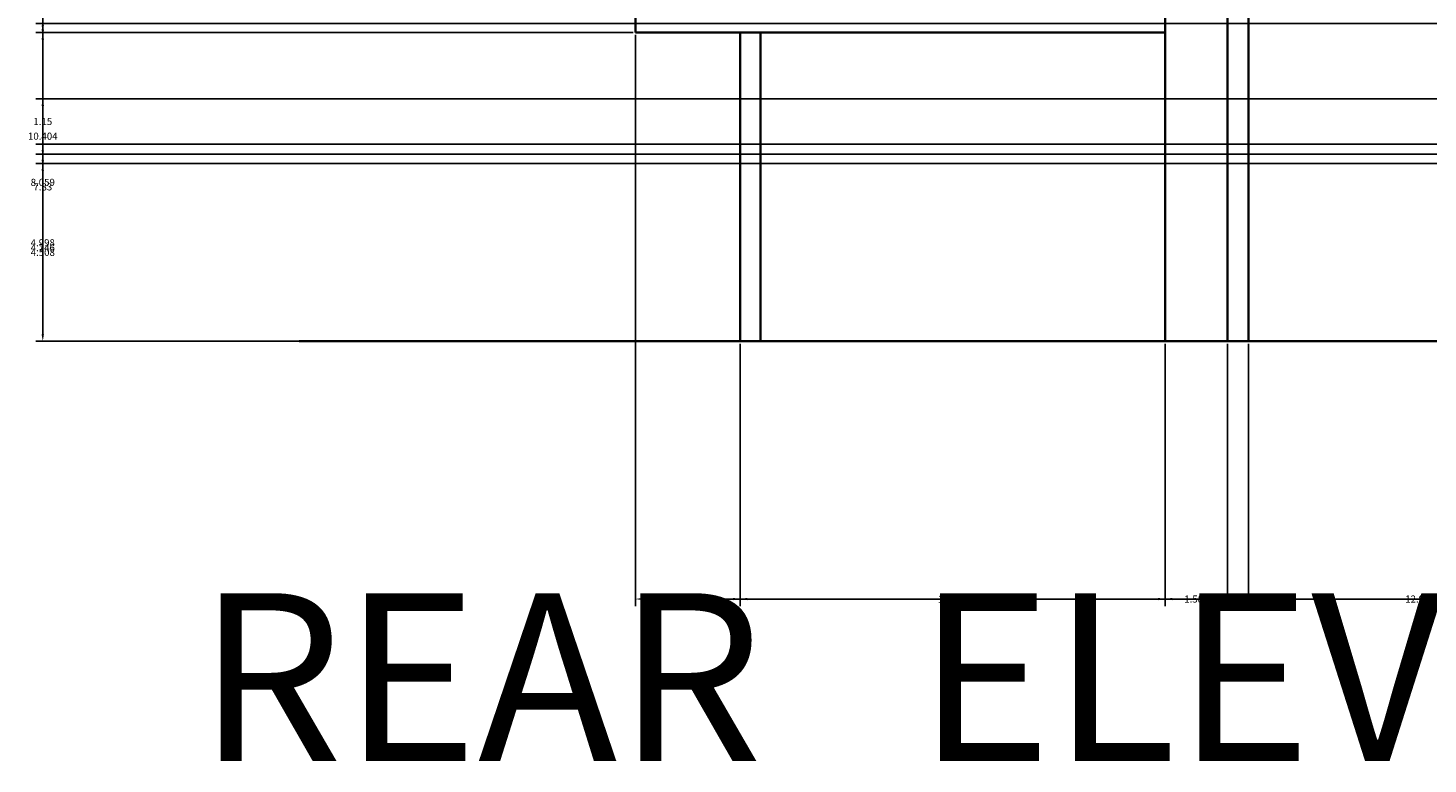
# Model space of a CAD drawing. Units: inches. Extents: x -10 to 130, y -32 to 34.
# Tile 1 of 22: x -10 to 26, y -32 to -13. Entities that reach past the tile are written whole.
import ezdxf

# ---------------------------------------------------------------- set-up
doc = ezdxf.new("R2010")
doc.units = ezdxf.units.IN
doc.header["$MEASUREMENT"] = 0
for name, color, linetype, lineweight in [('A-ANNO-DIMS', 2, 'Continuous', 18), ('A-ANNO-TEXT', 7, 'Continuous', 25), ('A-ELEV', 7, 'Continuous', 35)]:
    doc.layers.add(name, color=color, linetype=linetype, lineweight=lineweight)
doc.styles.get("Standard").update_dxf_attribs({"font": 'arial.ttf'})
doc.dimstyles.get("Standard").update_dxf_attribs({"dimtxt": 0.18, "dimasz": 0.18, "dimexe": 0.18, "dimexo": 0.0625, "dimgap": 0.09, "dimtad": 0, "dimtih": 1, "dimtoh": 1, "dimdec": 4, "dimzin": 0, "dimdsep": 46, "dimtxsty": 'Standard', "dimcen": 0.09, "dimadec": 0, "dimazin": 0, "dimtfac": 1, "dimtdec": 4, "dimtofl": 0, "dimtmove": 0, "dimatfit": 3, "dimfxl": 1, "dimtolj": 1, "dimtzin": 0, "dimarcsym": 0})

# ---------------------------------------------------------------- blocks, each defined once
blk = doc.blocks.new('*D1')
at = {"layer": 'A-ANNO-DIMS', "color": 0, "lineweight": -2, "transparency": 16777216}
for p, q in [((5.634, -13.647), (5.634, -28.129)), ((107.933, -21.477), (107.933, -28.129)), ((5.814, -27.949), (56.398, -27.949)), ((107.753, -27.949), (57.169, -27.949))]:
    blk.add_line(p, q, dxfattribs=at)
at = {"layer": 'A-ANNO-DIMS', "color": 0, "transparency": 16777216}
for points in [[(5.814, -27.919), (5.814, -27.979), (5.634, -27.949)], [(107.753, -27.919), (107.753, -27.979), (107.933, -27.949)]]:
    blk.add_solid(points, dxfattribs=at)
at = {"layer": 'Defpoints', "color": 0, "transparency": 16777216}
for p in [(5.634, -13.584), (107.933, -21.414), (107.933, -27.949)]:
    blk.add_point(p, dxfattribs=at)
at = {"layer": 'A-ANNO-DIMS', "color": 0, "transparency": 16777216, "insert": (56.784, -27.949), "char_height": 0.18, "attachment_point": 5}
blk.add_mtext('\\A1;102.3', dxfattribs=at)
blk = doc.blocks.new('*D30')
at = {"layer": 'A-ANNO-DIMS', "color": 0, "lineweight": -2, "transparency": 16777216}
for p, q in [((18.993, -11.011), (-9.564, -11.011)), ((-9.384, -11.191), (-9.384, -16.031)), ((-9.384, -21.234), (-9.384, -16.394)), ((8.226, -21.414), (-9.564, -21.414))]:
    blk.add_line(p, q, dxfattribs=at)
at = {"layer": 'A-ANNO-DIMS', "color": 0, "transparency": 16777216}
for points in [[(-9.414, -11.191), (-9.354, -11.191), (-9.384, -11.011)], [(-9.414, -21.234), (-9.354, -21.234), (-9.384, -21.414)]]:
    blk.add_solid(points, dxfattribs=at)
at = {"layer": 'Defpoints', "color": 0, "transparency": 16777216}
for p in [(-9.384, -11.011), (19.055, -11.011), (8.289, -21.414)]:
    blk.add_point(p, dxfattribs=at)
at = {"layer": 'A-ANNO-DIMS', "color": 0, "transparency": 16777216, "insert": (-9.384, -16.213), "char_height": 0.18, "attachment_point": 5}
blk.add_mtext('\\A1;10.404', dxfattribs=at)
blk = doc.blocks.new('*D40')
at = {"layer": 'A-ANNO-DIMS', "color": 0, "lineweight": -2, "transparency": 16777216}
for p, q in [((5.634, -13.647), (5.634, -28.129)), ((8.289, -21.477), (8.289, -28.129)), ((5.814, -27.949), (6.635, -27.949)), ((8.109, -27.949), (7.287, -27.949))]:
    blk.add_line(p, q, dxfattribs=at)
at = {"layer": 'A-ANNO-DIMS', "color": 0, "transparency": 16777216}
for points in [[(5.814, -27.919), (5.814, -27.979), (5.634, -27.949)], [(8.109, -27.919), (8.109, -27.979), (8.289, -27.949)]]:
    blk.add_solid(points, dxfattribs=at)
at = {"layer": 'Defpoints', "color": 0, "transparency": 16777216}
for p in [(5.634, -13.584), (8.289, -21.414), (8.289, -27.949)]:
    blk.add_point(p, dxfattribs=at)
at = {"layer": 'A-ANNO-DIMS', "color": 0, "transparency": 16777216, "insert": (6.961, -27.949), "char_height": 0.18, "attachment_point": 5}
blk.add_mtext('\\A1;2.65', dxfattribs=at)
blk = doc.blocks.new('*D41')
at = {"layer": 'A-ANNO-DIMS', "color": 0, "lineweight": -2, "transparency": 16777216}
for p, q in [((8.289, -21.477), (8.289, -28.129)), ((19.055, -21.477), (19.055, -28.129)), ((8.469, -27.949), (13.217, -27.949)), ((18.875, -27.949), (14.127, -27.949))]:
    blk.add_line(p, q, dxfattribs=at)
at = {"layer": 'A-ANNO-DIMS', "color": 0, "transparency": 16777216}
for points in [[(8.469, -27.919), (8.469, -27.979), (8.289, -27.949)], [(18.875, -27.919), (18.875, -27.979), (19.055, -27.949)]]:
    blk.add_solid(points, dxfattribs=at)
at = {"layer": 'Defpoints', "color": 0, "transparency": 16777216}
for p in [(8.289, -21.414), (19.055, -21.414), (19.055, -27.949)]:
    blk.add_point(p, dxfattribs=at)
at = {"layer": 'A-ANNO-DIMS', "color": 0, "transparency": 16777216, "insert": (13.672, -27.949), "char_height": 0.18, "attachment_point": 5}
blk.add_mtext('\\A1;10.766', dxfattribs=at)
blk = doc.blocks.new('*D42')
at = {"layer": 'A-ANNO-DIMS', "color": 0, "lineweight": -2, "transparency": 16777216}
for p, q in [((19.055, -21.477), (19.055, -28.129)), ((31.971, -21.477), (31.971, -28.129)), ((19.235, -27.949), (25.058, -27.949)), ((31.791, -27.949), (25.968, -27.949))]:
    blk.add_line(p, q, dxfattribs=at)
at = {"layer": 'A-ANNO-DIMS', "color": 0, "transparency": 16777216}
for points in [[(19.235, -27.919), (19.235, -27.979), (19.055, -27.949)], [(31.791, -27.919), (31.791, -27.979), (31.971, -27.949)]]:
    blk.add_solid(points, dxfattribs=at)
at = {"layer": 'Defpoints', "color": 0, "transparency": 16777216}
for p in [(19.055, -21.414), (31.971, -21.414), (31.971, -27.949)]:
    blk.add_point(p, dxfattribs=at)
at = {"layer": 'A-ANNO-DIMS', "color": 0, "transparency": 16777216, "insert": (25.513, -27.949), "char_height": 0.18, "attachment_point": 5}
blk.add_mtext('\\A1;12.916', dxfattribs=at)
blk = doc.blocks.new('*D45')
at = {"layer": 'A-ANNO-DIMS', "color": 0, "lineweight": -2, "transparency": 16777216}
for p, q in [((5.572, -13.584), (-9.564, -13.584)), ((-9.384, -13.764), (-9.384, -17.317)), ((-9.384, -21.234), (-9.384, -17.681)), ((8.226, -21.414), (-9.564, -21.414))]:
    blk.add_line(p, q, dxfattribs=at)
at = {"layer": 'A-ANNO-DIMS', "color": 0, "transparency": 16777216}
for points in [[(-9.414, -13.764), (-9.354, -13.764), (-9.384, -13.584)], [(-9.414, -21.234), (-9.354, -21.234), (-9.384, -21.414)]]:
    blk.add_solid(points, dxfattribs=at)
at = {"layer": 'Defpoints', "color": 0, "transparency": 16777216}
for p in [(-9.384, -13.584), (5.634, -13.584), (8.289, -21.414)]:
    blk.add_point(p, dxfattribs=at)
at = {"layer": 'A-ANNO-DIMS', "color": 0, "transparency": 16777216, "insert": (-9.384, -17.499), "char_height": 0.18, "attachment_point": 5}
blk.add_mtext('\\A1;7.83', dxfattribs=at)
blk = doc.blocks.new('*D46')
at = {"layer": 'A-ANNO-DIMS', "color": 0, "lineweight": -2, "transparency": 16777216}
for p, q in [((-9.384, -12.801), (-9.384, -12.621)), ((-9.384, -12.621), (-9.204, -12.621)), ((5.572, -12.801), (-9.564, -12.801)), ((-9.384, -13.404), (-9.384, -12.981)), ((5.572, -13.584), (-9.564, -13.584))]:
    blk.add_line(p, q, dxfattribs=at)
at = {"layer": 'A-ANNO-DIMS', "color": 0, "transparency": 16777216}
for points in [[(-9.414, -12.981), (-9.354, -12.981), (-9.384, -12.801)], [(-9.414, -13.404), (-9.354, -13.404), (-9.384, -13.584)]]:
    blk.add_solid(points, dxfattribs=at)
at = {"layer": 'Defpoints', "color": 0, "transparency": 16777216}
for p in [(-9.384, -12.801), (5.634, -12.801), (5.634, -13.584)]:
    blk.add_point(p, dxfattribs=at)
at = {"layer": 'A-ANNO-DIMS', "color": 0, "transparency": 16777216, "insert": (-8.81, -12.621), "char_height": 0.18, "attachment_point": 5}
blk.add_mtext('\\A1;0.783', dxfattribs=at)
blk = doc.blocks.new('*D49')
at = {"layer": 'A-ANNO-DIMS', "color": 0, "lineweight": -2, "transparency": 16777216}
for p, q in [((44.697, -13.356), (-9.564, -13.356)), ((-9.384, -13.536), (-9.384, -17.203)), ((-9.384, -21.234), (-9.384, -17.567)), ((44.697, -21.414), (-9.564, -21.414))]:
    blk.add_line(p, q, dxfattribs=at)
at = {"layer": 'A-ANNO-DIMS', "color": 0, "transparency": 16777216}
for points in [[(-9.414, -13.536), (-9.354, -13.536), (-9.384, -13.356)], [(-9.414, -21.234), (-9.354, -21.234), (-9.384, -21.414)]]:
    blk.add_solid(points, dxfattribs=at)
at = {"layer": 'Defpoints', "color": 0, "transparency": 16777216}
for p in [(44.76, -13.356), (-9.384, -21.414), (44.76, -21.414)]:
    blk.add_point(p, dxfattribs=at)
at = {"layer": 'A-ANNO-DIMS', "color": 0, "transparency": 16777216, "insert": (-9.384, -17.385), "char_height": 0.18, "attachment_point": 5}
blk.add_mtext('\\A1;8.059', dxfattribs=at)
blk = doc.blocks.new('*D64')
at = {"layer": 'A-ANNO-DIMS', "color": 0, "lineweight": -2, "transparency": 16777216}
for p, q in [((82.315, -15.264), (-9.564, -15.264)), ((-9.384, -15.444), (-9.384, -15.659)), ((-9.384, -16.237), (-9.384, -16.022)), ((82.315, -16.417), (-9.564, -16.417))]:
    blk.add_line(p, q, dxfattribs=at)
at = {"layer": 'A-ANNO-DIMS', "color": 0, "transparency": 16777216}
for points in [[(-9.414, -15.444), (-9.354, -15.444), (-9.384, -15.264)], [(-9.414, -16.237), (-9.354, -16.237), (-9.384, -16.417)]]:
    blk.add_solid(points, dxfattribs=at)
at = {"layer": 'Defpoints', "color": 0, "transparency": 16777216}
for p in [(82.377, -15.264), (-9.384, -16.417), (82.377, -16.417)]:
    blk.add_point(p, dxfattribs=at)
at = {"layer": 'A-ANNO-DIMS', "color": 0, "transparency": 16777216, "insert": (-9.384, -15.841), "char_height": 0.18, "attachment_point": 5}
blk.add_mtext('\\A1;1.15', dxfattribs=at)
blk = doc.blocks.new('*D65')
at = {"layer": 'A-ANNO-DIMS', "color": 0, "lineweight": -2, "transparency": 16777216}
for p, q in [((82.315, -16.417), (-9.564, -16.417)), ((-9.384, -16.597), (-9.384, -18.734)), ((-9.384, -21.234), (-9.384, -19.097)), ((80.669, -21.414), (-9.564, -21.414))]:
    blk.add_line(p, q, dxfattribs=at)
at = {"layer": 'A-ANNO-DIMS', "color": 0, "transparency": 16777216}
for points in [[(-9.414, -16.597), (-9.354, -16.597), (-9.384, -16.417)], [(-9.414, -21.234), (-9.354, -21.234), (-9.384, -21.414)]]:
    blk.add_solid(points, dxfattribs=at)
at = {"layer": 'Defpoints', "color": 0, "transparency": 16777216}
for p in [(-9.384, -16.417), (82.377, -16.417), (80.731, -21.414)]:
    blk.add_point(p, dxfattribs=at)
at = {"layer": 'A-ANNO-DIMS', "color": 0, "transparency": 16777216, "insert": (-9.384, -18.916), "char_height": 0.18, "attachment_point": 5}
blk.add_mtext('\\A1;4.998', dxfattribs=at)
blk = doc.blocks.new('*D69')
at = {"layer": 'A-ANNO-DIMS', "color": 0, "lineweight": -2, "transparency": 16777216}
for p, q in [((89.095, -16.906), (-9.564, -16.906)), ((-9.384, -17.086), (-9.384, -18.979)), ((-9.384, -21.234), (-9.384, -19.342)), ((89.095, -21.414), (-9.564, -21.414))]:
    blk.add_line(p, q, dxfattribs=at)
at = {"layer": 'A-ANNO-DIMS', "color": 0, "transparency": 16777216}
for points in [[(-9.414, -17.086), (-9.354, -17.086), (-9.384, -16.906)], [(-9.414, -21.234), (-9.354, -21.234), (-9.384, -21.414)]]:
    blk.add_solid(points, dxfattribs=at)
at = {"layer": 'Defpoints', "color": 0, "transparency": 16777216}
for p in [(89.158, -16.906), (-9.384, -21.414), (89.158, -21.414)]:
    blk.add_point(p, dxfattribs=at)
at = {"layer": 'A-ANNO-DIMS', "color": 0, "transparency": 16777216, "insert": (-9.384, -19.16), "char_height": 0.18, "attachment_point": 5}
blk.add_mtext('\\A1;4.508', dxfattribs=at)
blk = doc.blocks.new('*D132')
at = {"layer": 'A-ANNO-DIMS', "color": 0, "lineweight": -2, "transparency": 16777216}
for p, q in [((19.055, -21.477), (19.055, -28.129)), ((20.637, -21.477), (20.637, -28.129)), ((19.235, -27.949), (19.478, -27.949)), ((20.457, -27.949), (20.214, -27.949))]:
    blk.add_line(p, q, dxfattribs=at)
at = {"layer": 'A-ANNO-DIMS', "color": 0, "transparency": 16777216}
for points in [[(19.235, -27.919), (19.235, -27.979), (19.055, -27.949)], [(20.457, -27.919), (20.457, -27.979), (20.637, -27.949)]]:
    blk.add_solid(points, dxfattribs=at)
at = {"layer": 'Defpoints', "color": 0, "transparency": 16777216}
for p in [(19.055, -21.414), (20.637, -21.414), (20.637, -27.949)]:
    blk.add_point(p, dxfattribs=at)
at = {"layer": 'A-ANNO-DIMS', "color": 0, "transparency": 16777216, "insert": (19.846, -27.949), "char_height": 0.18, "attachment_point": 5}
blk.add_mtext('\\A1;1.581', dxfattribs=at)
blk = doc.blocks.new('*D133')
at = {"layer": 'A-ANNO-DIMS', "color": 0, "lineweight": -2, "transparency": 16777216}
for p, q in [((20.637, -21.477), (20.637, -28.129)), ((21.169, -21.477), (21.169, -28.129)), ((20.457, -27.949), (20.277, -27.949)), ((21.349, -27.949), (21.529, -27.949))]:
    blk.add_line(p, q, dxfattribs=at)
at = {"layer": 'A-ANNO-DIMS', "color": 0, "transparency": 16777216}
for points in [[(20.457, -27.919), (20.457, -27.979), (20.637, -27.949)], [(21.349, -27.919), (21.349, -27.979), (21.169, -27.949)]]:
    blk.add_solid(points, dxfattribs=at)
at = {"layer": 'Defpoints', "color": 0, "transparency": 16777216}
for p in [(20.637, -21.414), (21.169, -21.414), (21.169, -27.949)]:
    blk.add_point(p, dxfattribs=at)
at = {"layer": 'A-ANNO-DIMS', "color": 0, "transparency": 16777216, "insert": (21.922, -27.949), "char_height": 0.18, "attachment_point": 5}
blk.add_mtext('\\A1;0.532', dxfattribs=at)
blk = doc.blocks.new('*D135')
at = {"layer": 'A-ANNO-DIMS', "color": 0, "lineweight": -2, "transparency": 16777216}
for p, q in [((26.306, -16.668), (-9.564, -16.668)), ((-9.384, -16.848), (-9.384, -18.859)), ((-9.384, -21.234), (-9.384, -19.223)), ((26.306, -21.414), (-9.564, -21.414))]:
    blk.add_line(p, q, dxfattribs=at)
at = {"layer": 'A-ANNO-DIMS', "color": 0, "transparency": 16777216}
for points in [[(-9.414, -16.848), (-9.354, -16.848), (-9.384, -16.668)], [(-9.414, -21.234), (-9.354, -21.234), (-9.384, -21.414)]]:
    blk.add_solid(points, dxfattribs=at)
at = {"layer": 'Defpoints', "color": 0, "transparency": 16777216}
for p in [(26.368, -16.668), (-9.384, -21.414), (26.368, -21.414)]:
    blk.add_point(p, dxfattribs=at)
at = {"layer": 'A-ANNO-DIMS', "color": 0, "transparency": 16777216, "insert": (-9.384, -19.041), "char_height": 0.18, "attachment_point": 5}
blk.add_mtext('\\A1;4.746', dxfattribs=at)

msp = doc.modelspace()

# ---------------------------------------------------------------- linework, layer by layer
at = {"layer": 'A-ELEV'}
for p, q in [((20.6365, -6.2218), (20.6365, -16.1883)), ((21.1687, -6.2218), (21.1687, -16.1883)), ((19.055, -21.4145), (19.055, -11.0106)), ((5.634, -12.8012), (5.634, -13.5841)), ((5.634, -13.5841), (19.055, -13.5841)), ((8.2886, -13.5841), (8.2886, -21.4145)), ((8.8031, -13.5841), (8.8031, -21.4145)), ((20.6365, -16.1883), (20.6365, -21.4145)), ((21.1687, -16.1883), (21.1687, -21.4145)), ((21.1687, -21.4145), (-2.8836, -21.4145)), ((31.9712, -21.4145), (21.1687, -21.4145))]:
    msp.add_line(p, q, dxfattribs=at)

# ---------------------------------------------------------------- texts
at = {"layer": 'A-ANNO-TEXT'}
msp.add_text('REAR   ELEVATION    AND   LOGISTICS   HUB', height=4.256275, dxfattribs=at).set_placement((-5.4651, -32.0569))

# ---------------------------------------------------------------- dimensions: what is measured, and where the dimension line sits
at = {"layer": 'A-ANNO-DIMS'}
for base, p1, p2, override, picture, middle in [((-9.3836, -11.0106), (8.2886, -21.4145), (19.055, -11.0106), {"dimdec": 3, "dimlfac": 1, "dimrnd": 0, "dimzin": 0, "dimdsep": 46, "dimlunit": 2}, '*D30', (-9.3836, -16.2125)), ((-9.3836, -12.8012), (5.634, -13.5841), (5.634, -12.8012), {"dimdec": 3, "dimlfac": 1, "dimrnd": 0, "dimzin": 0, "dimdsep": 46, "dimlunit": 2}, '*D46', (-8.8098, -12.6212)), ((-9.3836, -21.4145), (44.76, -13.3558), (44.76, -21.4145), {"dimdec": 3, "dimlfac": 1, "dimrnd": 0, "dimzin": 0, "dimdsep": 46, "dimlunit": 2}, '*D49', (-9.3836, -17.3852)), ((-9.3836, -13.5841), (8.2886, -21.4145), (5.634, -13.5841), {"dimdec": 2, "dimlfac": 1, "dimrnd": 0, "dimzin": 0, "dimdsep": 46, "dimlunit": 2}, '*D45', (-9.3836, -17.4993)), ((-9.3836, -16.4166), (82.377, -15.2645), (82.377, -16.4166), {"dimdec": 2, "dimlfac": 1, "dimrnd": 0, "dimzin": 0, "dimdsep": 46, "dimlunit": 2}, '*D64', (-9.3836, -15.8406)), ((-9.3836, -16.4166), (80.7314, -21.4145), (82.377, -16.4166), {"dimdec": 3, "dimlfac": 1, "dimrnd": 0, "dimzin": 0, "dimdsep": 46, "dimlunit": 2}, '*D65', (-9.3836, -18.9156)), ((-9.38355, -21.41449), (26.36827, -16.66804), (26.36827, -21.41449), {"dimdec": 3, "dimlfac": 1, "dimrnd": 0, "dimzin": 0, "dimdsep": 46, "dimlunit": 2}, '*D135', (-9.38355, -19.04127)), ((-9.3836, -21.4145), (89.1578, -16.9063), (89.1578, -21.4145), {"dimdec": 3, "dimlfac": 1, "dimrnd": 0, "dimzin": 0, "dimdsep": 46, "dimlunit": 2}, '*D69', (-9.3836, -19.1604))]:
    dim = msp.add_linear_dim(base=base, p1=p1, p2=p2, angle=90, dimstyle='Standard', override=override, dxfattribs=at)
    dim.commit()
    dim.dimension.update_dxf_attribs({"geometry": picture, "text_midpoint": middle})
for base, p1, p2, override, picture, middle in [((107.9333, -27.9493), (5.634, -13.5841), (107.9333, -21.4145), {"dimdec": 1, "dimlfac": 1, "dimrnd": 0, "dimzin": 0, "dimdsep": 46, "dimlunit": 2}, '*D1', (56.7837, -27.9493)), ((8.2886, -27.9493), (5.634, -13.5841), (8.2886, -21.4145), {"dimdec": 2, "dimlfac": 1, "dimrnd": 0, "dimzin": 0, "dimdsep": 46, "dimlunit": 2}, '*D40', (6.9613, -27.9493)), ((19.055, -27.9493), (8.2886, -21.4145), (19.055, -21.4145), {"dimdec": 3, "dimlfac": 1, "dimrnd": 0, "dimzin": 0, "dimdsep": 46, "dimlunit": 2}, '*D41', (13.6718, -27.9493)), ((31.9712, -27.9493), (19.055, -21.4145), (31.9712, -21.4145), {"dimdec": 3, "dimlfac": 1, "dimrnd": 0, "dimzin": 0, "dimdsep": 46, "dimlunit": 2}, '*D42', (25.5131, -27.9493)), ((20.63651, -27.9493), (19.05502, -21.41449), (20.63651, -21.41449), {"dimdec": 3, "dimlfac": 1, "dimrnd": 0, "dimzin": 0, "dimdsep": 46, "dimlunit": 2}, '*D132', (19.84577, -27.9493)), ((21.1687, -27.9493), (20.6365, -21.4145), (21.1687, -21.4145), {"dimdec": 3, "dimlfac": 1, "dimrnd": 0, "dimzin": 0, "dimdsep": 46, "dimlunit": 2}, '*D133', (21.9215, -27.9493))]:
    dim = msp.add_linear_dim(base=base, p1=p1, p2=p2, dimstyle='Standard', override=override, dxfattribs=at)
    dim.commit()
    dim.dimension.update_dxf_attribs({"geometry": picture, "text_midpoint": middle})

doc.saveas('drawing.dxf')
